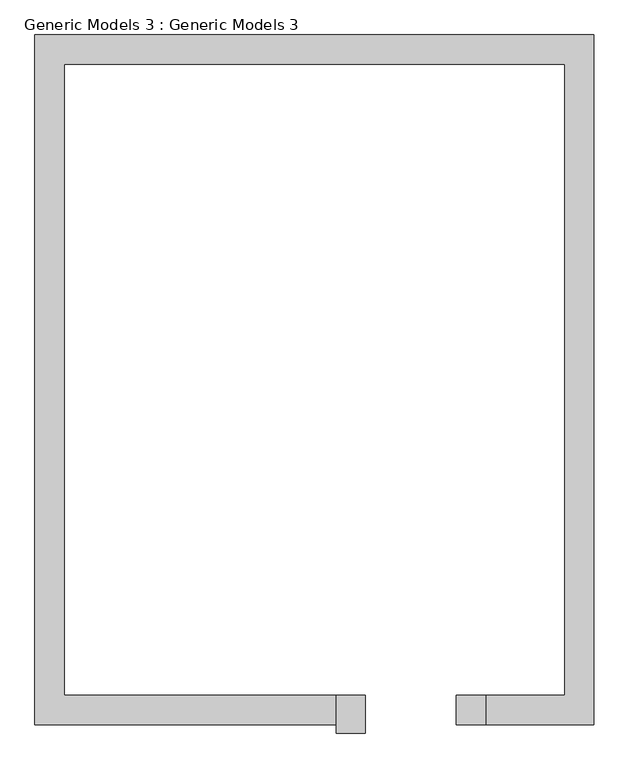
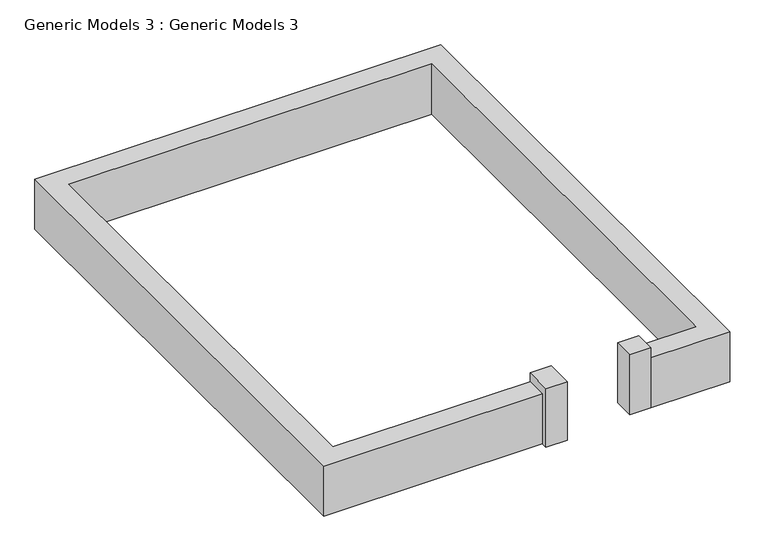
"""IFC4 building model written with IfcOpenShell, lengths in millimetres: proxy geometry, Generic Models 3 : Generic Models 3."""

from ifc_helpers import new_model, si_unit, frame, origin, place, context, project, spatial, polyline, outline, extrude, source, transform, mapped, element, save


def generic_models_3_generic_models_3_c69b0eb2(model_context):
    return source(origin(), model_context, "Body", "SweptSolid", [
        extrude(outline(polyline([(-10060.5094994, -18172.6805842), (-10060.5094994, -17258.2805842), (-9146.1094994, -17258.2805842), (-9146.1094994, -18172.6805842), (-10060.5094994, -18172.6805842)])), frame((0.0, 0.0, -304.8), z_axis=(0.0, 0.0, 1.0), x_axis=(1.0, 0.0, 0.0)), (0.0, 0.0, 1.0), 2734.9873422),
        extrude(outline(polyline([(-9146.1094994, -17258.2805842), (-6669.6094994, -17258.2805842), (-6669.6094994, 2512.5006048), (-22349.7112937, 2512.5006048), (-22349.7112937, -17258.2805842), (-13832.4094994, -17258.2805842), (-13832.4094994, -18172.6805842), (-23264.1112937, -18172.6805842), (-23264.1112937, 3426.9006048), (-5755.2094994, 3426.9006048), (-5755.2094994, -18172.6805842), (-9146.1094994, -18172.6805842), (-9146.1094994, -17258.2805842)])), frame((0.0, 0.0, -304.8), z_axis=(0.0, 0.0, 1.0), x_axis=(1.0, 0.0, 0.0)), (0.0, 0.0, 1.0), 2288.9904797),
        extrude(outline(polyline([(-12918.0094994, -17258.2805842), (-12918.0094994, -18439.3805842), (-13832.4094994, -18439.3805842), (-13832.4094994, -17258.2805842), (-12918.0094994, -17258.2805842)])), frame((0.0, 0.0, -304.8), z_axis=(0.0, 0.0, 1.0), x_axis=(1.0, 0.0, 0.0)), (0.0, 0.0, 1.0), 2686.8013914),
    ])


if __name__ == "__main__":
    model = new_model("IFC4")
    model_context = context("Model", 3, world=origin())
    ifc_project = project(units=[si_unit("LENGTHUNIT", "METRE", prefix="MILLI")], contexts=[model_context])
    site = spatial("IfcSite", under=ifc_project)
    building = spatial("IfcBuilding", under=site)
    placement = place(None, origin())
    generic_models_3_generic_models_3_shape = generic_models_3_generic_models_3_c69b0eb2(model_context)
    element("IfcBuildingElementProxy", 1, Name="Generic Models 3 : Generic Models 3", ObjectType="Generic Models 3 : Generic Models 3", at=placement, inside=building, context=model_context, shape_type="MappedRepresentation", body=[
        mapped(generic_models_3_generic_models_3_shape, transform((0.0, 0.0, 0.0), x_axis=(1.0, 0.0, 0.0), y_axis=(0.0, 1.0, 0.0), z_axis=(0.0, 0.0, 1.0))),
    ])
    save(model, "model.ifc")
